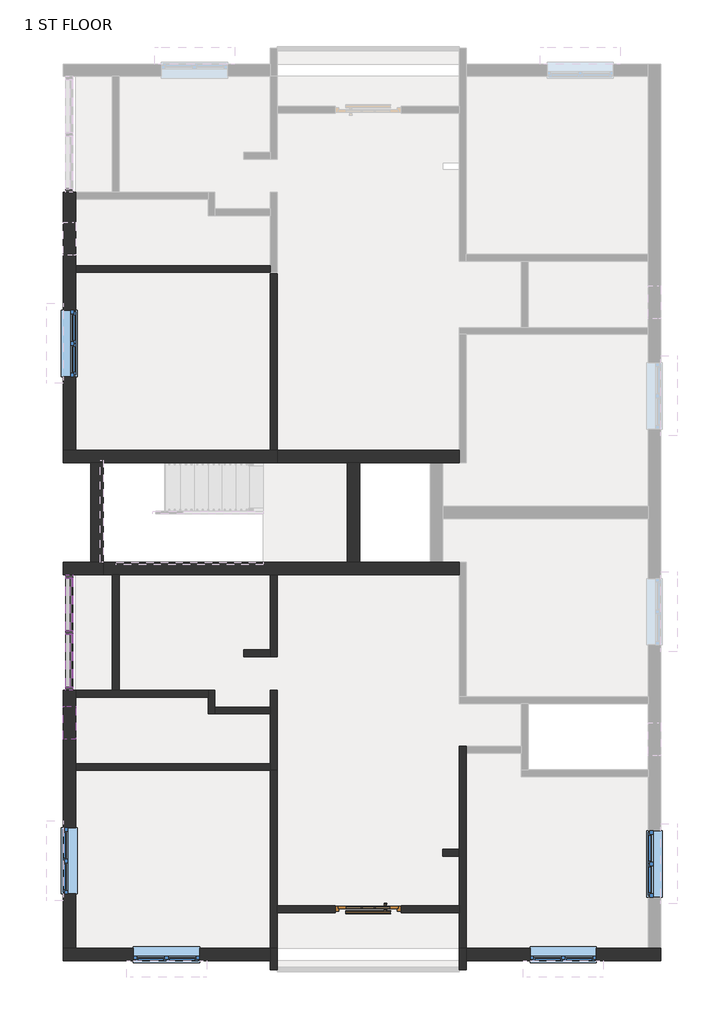
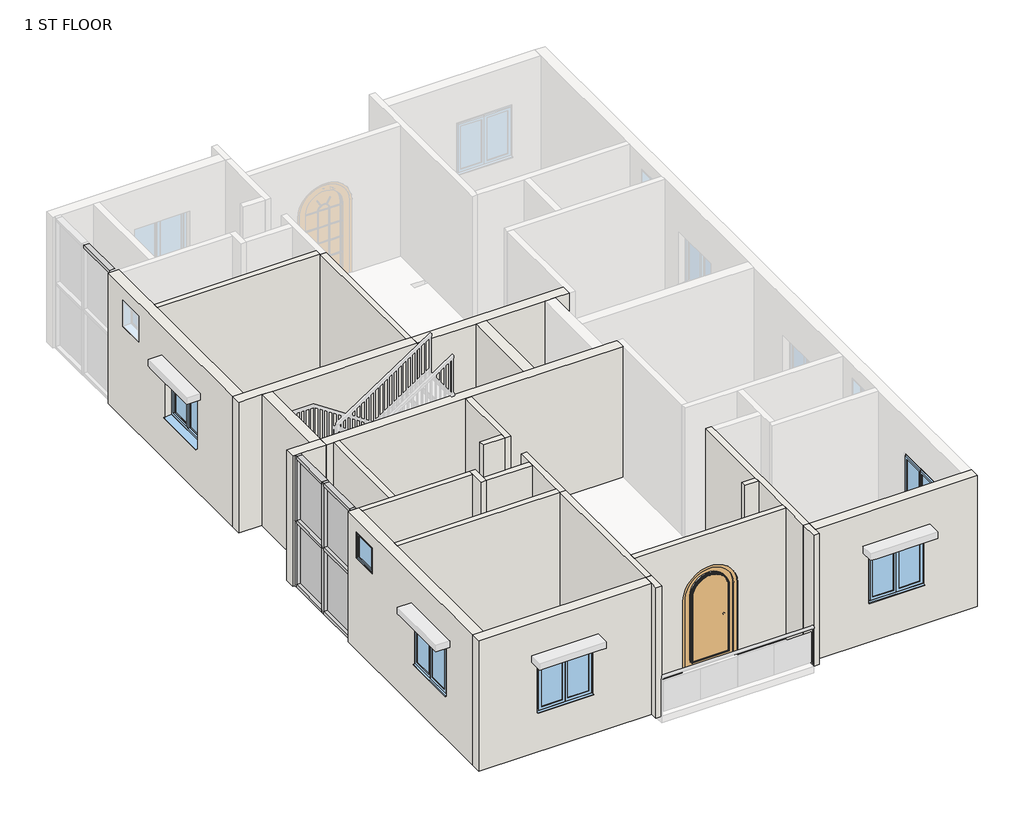
# One storey, part 1 of 4: 26 walls, 14 members, 6 windows, 4 plates, 1 door.
"""IFC4 building model written with IfcOpenShell, lengths in millimetres."""

from ifc_helpers import new_model, si_unit, point, frame, frame_2d, origin, place, context, project, spatial, polyline, circle_curve, trimmed, segment, composite_curve, outline, extrude, faceted_brep, transform, mapped, element, save
from components import door_arched_single_french_glass_wood_exterior_4_x_7_french_5c4dec95, member_801a2072, member_82905deb, member_88aa5c81, member_4491d118, system_panel_glazed_a8655be6, window_80340324, w2_windows_4_x_4_9dec5fc7

model = new_model("IFC4")

# Units and contexts
model_context = context("Model", 3, world=origin())
ifc_project = project(units=[si_unit("LENGTHUNIT", "METRE", prefix="MILLI")], contexts=[model_context])

# Site, building, storey
site = spatial("IfcSite", under=ifc_project)
building = spatial("IfcBuilding", under=site)
storey = spatial("IfcBuildingStorey", under=building, Name="1 ST FLOOR", Elevation=6096.0)

# Door
placement = place(None, origin())
door_arched_single_french_glass_wood_exterior_4_x_7_french_shape = door_arched_single_french_glass_wood_exterior_4_x_7_french_5c4dec95(model_context)
element("IfcDoor", 1, ObjectType="Door_Arched_Single_French_Glass_Wood_Exterior : 4' x 7' french door", at=placement, inside=storey, context=model_context, shape_type="MappedRepresentation", body=[
    mapped(door_arched_single_french_glass_wood_exterior_4_x_7_french_shape, transform((-817.6012202, -2286.2690997, 6096.0), x_axis=(-1.0, 0.0, 0.0), y_axis=(0.0, -1.0, 0.0), z_axis=(0.0, 0.0, 1.0))),
])

# Members
member_shape = member_801a2072(model_context)
element("IfcMember", 2, ObjectType="Rectangular Mullion : 2.5\" x 5\" rectangular", at=placement, inside=storey, context=model_context, shape_type="MappedRepresentation", body=[
    mapped(member_shape, transform((-6318.2887202, 10972.5309003, 9144.0), x_axis=(0.0, 0.0, 1.0), y_axis=(-1.0, 0.0, 0.0), z_axis=(0.0, -1.0, 0.0))),
])
element("IfcMember", 3, ObjectType="Rectangular Mullion : 2.5\" x 5\" rectangular", at=placement, inside=storey, context=model_context, shape_type="MappedRepresentation", body=[
    mapped(member_shape, transform((-6318.2887202, 1803.1309003, 9144.0), x_axis=(0.0, 0.0, 1.0), y_axis=(-1.0, 0.0, 0.0), z_axis=(0.0, -1.0, 0.0))),
])
element("IfcMember", 4, ObjectType="Rectangular Mullion : 2.5\" x 5\" rectangular", at=placement, inside=storey, context=model_context, shape_type="MappedRepresentation", body=[
    mapped(member_shape, transform((-6318.2887202, 2838.1809003, 9144.0), x_axis=(0.0, 0.0, 1.0), y_axis=(-1.0, 0.0, 0.0), z_axis=(0.0, -1.0, 0.0))),
])
element("IfcMember", 5, ObjectType="Rectangular Mullion : 2.5\" x 5\" rectangular", at=placement, inside=storey, context=model_context, shape_type="MappedRepresentation", body=[
    mapped(member_shape, transform((-6318.2887202, 3809.7309003, 6096.0), x_axis=(0.0, 0.0, -1.0), y_axis=(-1.0, 0.0, 0.0), z_axis=(0.0, 1.0, 0.0))),
])
element("IfcMember", 6, ObjectType="Rectangular Mullion : 2.5\" x 5\" rectangular", at=placement, inside=storey, context=model_context, shape_type="MappedRepresentation", body=[
    mapped(member_shape, transform((-6318.2887202, 2774.6809003, 6096.0), x_axis=(0.0, 0.0, -1.0), y_axis=(-1.0, 0.0, 0.0), z_axis=(0.0, 1.0, 0.0))),
])
member_2_shape = member_82905deb(model_context)
element("IfcMember", 7, ObjectType="Rectangular Mullion : 2.5\" x 5\" rectangular", at=placement, inside=storey, context=model_context, shape_type="MappedRepresentation", body=[
    mapped(member_2_shape, transform((-6318.2887202, 2806.4309003, 6096.0), x_axis=(0.0, -1.0, 0.0), y_axis=(-1.0, 0.0, 0.0), z_axis=(0.0, 0.0, -1.0))),
])
member_3_shape = member_88aa5c81(model_context)
element("IfcMember", 8, ObjectType="Rectangular Mullion : 2.5\" x 5\" rectangular", at=placement, inside=storey, context=model_context, shape_type="MappedRepresentation", body=[
    mapped(member_3_shape, transform((-6318.2887202, 2838.1809003, 7620.0), x_axis=(0.0, 0.0, 1.0), y_axis=(-1.0, 0.0, 0.0), z_axis=(0.0, -1.0, 0.0))),
])
element("IfcMember", 9, ObjectType="Rectangular Mullion : 2.5\" x 5\" rectangular", at=placement, inside=storey, context=model_context, shape_type="MappedRepresentation", body=[
    mapped(member_3_shape, transform((-6318.2887202, 1803.1309003, 7620.0), x_axis=(0.0, 0.0, 1.0), y_axis=(-1.0, 0.0, 0.0), z_axis=(0.0, -1.0, 0.0))),
])
element("IfcMember", 10, ObjectType="Rectangular Mullion : 2.5\" x 5\" rectangular", at=placement, inside=storey, context=model_context, shape_type="MappedRepresentation", body=[
    mapped(member_2_shape, transform((-6318.2887202, 2806.4309003, 7620.0), x_axis=(0.0, -1.0, 0.0), y_axis=(-1.0, 0.0, 0.0), z_axis=(0.0, 0.0, -1.0))),
])
member_4_shape = member_4491d118(model_context)
element("IfcMember", 11, ObjectType="Rectangular Mullion : 2.5\" x 5\" rectangular", at=placement, inside=storey, context=model_context, shape_type="MappedRepresentation", body=[
    mapped(member_4_shape, transform((-6318.2887202, 10909.0309003, 6096.0), x_axis=(0.0, -1.0, 0.0), y_axis=(-1.0, 0.0, 0.0), z_axis=(0.0, 0.0, -1.0))),
])
element("IfcMember", 12, ObjectType="Rectangular Mullion : 2.5\" x 5\" rectangular", at=placement, inside=storey, context=model_context, shape_type="MappedRepresentation", body=[
    mapped(member_4_shape, transform((-6318.2887202, 1739.6309003, 6096.0), x_axis=(0.0, -1.0, 0.0), y_axis=(-1.0, 0.0, 0.0), z_axis=(0.0, 0.0, -1.0))),
])
element("IfcMember", 13, ObjectType="Rectangular Mullion : 2.5\" x 5\" rectangular", at=placement, inside=storey, context=model_context, shape_type="MappedRepresentation", body=[
    mapped(member_4_shape, transform((-6318.2887202, 3873.2309003, 9144.0), x_axis=(0.0, 1.0, 0.0), y_axis=(-1.0, 0.0, 0.0), z_axis=(0.0, 0.0, 1.0))),
])
element("IfcMember", 14, ObjectType="Rectangular Mullion : 2.5\" x 5\" rectangular", at=placement, inside=storey, context=model_context, shape_type="MappedRepresentation", body=[
    mapped(member_4_shape, transform((-6318.2887202, 1739.6309003, 7620.0), x_axis=(0.0, -1.0, 0.0), y_axis=(-1.0, 0.0, 0.0), z_axis=(0.0, 0.0, -1.0))),
])
element("IfcMember", 15, ObjectType="Rectangular Mullion : 2.5\" x 5\" rectangular", at=placement, inside=storey, context=model_context, shape_type="MappedRepresentation", body=[
    mapped(member_4_shape, transform((-6318.2887202, 3873.2309003, 7620.0), x_axis=(0.0, 1.0, 0.0), y_axis=(-1.0, 0.0, 0.0), z_axis=(0.0, 0.0, 1.0))),
])

# Plates
system_panel_glazed_shape = system_panel_glazed_a8655be6(model_context)
element("IfcPlate", 16, ObjectType="System Panel : Glazed", at=placement, inside=storey, context=model_context, shape_type="MappedRepresentation", body=[
    mapped(system_panel_glazed_shape, transform((-6318.2887202, 3323.9559003, 6159.5), x_axis=(0.0, -1.0, 0.0), y_axis=(1.0, 0.0, 0.0), z_axis=(0.0, 0.0, 1.0))),
])
element("IfcPlate", 17, ObjectType="System Panel : Glazed", at=placement, inside=storey, context=model_context, shape_type="MappedRepresentation", body=[
    mapped(system_panel_glazed_shape, transform((-6318.2887202, 2288.9059003, 6159.5), x_axis=(0.0, -1.0, 0.0), y_axis=(1.0, 0.0, 0.0), z_axis=(0.0, 0.0, 1.0))),
])
element("IfcPlate", 18, ObjectType="System Panel : Glazed", at=placement, inside=storey, context=model_context, shape_type="MappedRepresentation", body=[
    mapped(system_panel_glazed_shape, transform((-6318.2887202, 3323.9559003, 7651.75), x_axis=(0.0, -1.0, 0.0), y_axis=(1.0, 0.0, 0.0), z_axis=(0.0, 0.0, 1.0))),
])
element("IfcPlate", 19, ObjectType="System Panel : Glazed", at=placement, inside=storey, context=model_context, shape_type="MappedRepresentation", body=[
    mapped(system_panel_glazed_shape, transform((-6318.2887202, 2288.9059003, 7651.75), x_axis=(0.0, -1.0, 0.0), y_axis=(1.0, 0.0, 0.0), z_axis=(0.0, 0.0, 1.0))),
])

# Walls
element("IfcWall", 20, ObjectType="OUTER WALL 9\"", at=placement, inside=storey, context=model_context, shape_type="Brep", body=[
    faceted_brep([(-6432.5887202, -3238.7690997, 6096.0), (-2621.0012202, -3238.7690997, 6096.0), (-2621.0012202, -3238.7690997, 9144.0), (-6432.5887202, -3238.7690997, 9144.0), (-5137.1887202, -3238.7690997, 7010.4), (-5137.1887202, -3238.7690997, 8229.6), (-3917.9887202, -3238.7690997, 8229.6), (-3917.9887202, -3238.7690997, 7010.4), (-6432.5887202, -3010.1690997, 6096.0), (-6432.5887202, -3010.1690997, 9144.0), (-6203.9887202, -3010.1690997, 9144.0), (-2621.0012202, -3010.1690997, 9144.0), (-2621.0012202, -3010.1690997, 6096.0), (-6203.9887202, -3010.1690997, 6096.0), (-5137.1887202, -3010.1690997, 7010.4), (-3917.9887202, -3010.1690997, 7010.4), (-3917.9887202, -3010.1690997, 8229.6), (-5137.1887202, -3010.1690997, 8229.6)], [[[0, 1, 2, 3], [4, 5, 6, 7]], [[8, 9, 10, 11, 12, 13], [14, 15, 16, 17]], [[1, 0, 8, 13, 12]], [[3, 2, 11, 10, 9]], [[0, 3, 9, 8]], [[2, 1, 12, 11]], [[5, 4, 14, 17]], [[6, 5, 17, 16]], [[7, 6, 16, 15]], [[4, 7, 15, 14]]]),
])
element("IfcWall", 21, ObjectType="OUTER WALL 9\"", at=placement, inside=storey, context=model_context, shape_type="Brep", body=[
    faceted_brep([(-6203.9887202, -3010.1690997, 9144.0), (-6203.9887202, -3010.1690997, 6096.0), (-6203.9887202, 266.4309003, 6096.0), (-6203.9887202, 393.4309003, 6096.0), (-6203.9887202, 1612.6309003, 6096.0), (-6203.9887202, 1739.6309003, 6096.0), (-6203.9887202, 1739.6309003, 9144.0), (-6203.9887202, 1612.6309003, 9144.0), (-6203.9887202, 393.4309003, 9144.0), (-6203.9887202, 266.4309003, 9144.0), (-6203.9887202, -787.6690997, 7096.0), (-6203.9887202, -2006.8690997, 7096.0), (-6203.9887202, -2006.8690997, 8315.2), (-6203.9887202, -787.6690997, 8315.2), (-6203.9887202, 1447.5309003, 8839.2), (-6203.9887202, 1447.5309003, 8229.6), (-6203.9887202, 837.9309003, 8229.6), (-6203.9887202, 837.9309003, 8839.2), (-6432.5887202, -3010.1690997, 6096.0), (-6432.5887202, -3010.1690997, 9144.0), (-6432.5887202, 1739.6309003, 9144.0), (-6432.5887202, 1739.6309003, 6096.0), (-6432.5887202, -787.6690997, 7096.0), (-6432.5887202, -787.6690997, 8315.2), (-6432.5887202, -2006.8690997, 8315.2), (-6432.5887202, -2006.8690997, 7096.0), (-6432.5887202, 1447.5309003, 8839.2), (-6432.5887202, 837.9309003, 8839.2), (-6432.5887202, 837.9309003, 8229.6), (-6432.5887202, 1447.5309003, 8229.6)], [[[0, 1, 2, 3, 4, 5, 6, 7, 8, 9], [10, 11, 12, 13], [14, 15, 16, 17]], [[18, 19, 20, 21], [22, 23, 24, 25], [26, 27, 28, 29]], [[1, 18, 21, 5, 4, 3, 2]], [[19, 0, 9, 8, 7, 6, 20]], [[1, 0, 19, 18]], [[6, 5, 21, 20]], [[23, 22, 10, 13]], [[24, 23, 13, 12]], [[25, 24, 12, 11]], [[22, 25, 11, 10]], [[15, 14, 26, 29]], [[16, 15, 29, 28]], [[17, 16, 28, 27]], [[14, 17, 27, 26]]]),
])
element("IfcWall", 22, ObjectType="OUTER WALL 9\"", at=placement, inside=storey, context=model_context, shape_type="Brep", body=[
    faceted_brep([(4567.1987798, -3010.1690997, 6096.0), (4338.5987798, -3010.1690997, 6096.0), (985.7987798, -3010.1690997, 6096.0), (985.7987798, -3010.1690997, 9144.0), (4338.5987798, -3010.1690997, 9144.0), (4567.1987798, -3010.1690997, 9144.0), (2166.8987798, -3010.1690997, 7010.4), (3386.0987798, -3010.1690997, 7010.4), (3386.0987798, -3010.1690997, 8229.6), (2166.8987798, -3010.1690997, 8229.6), (4567.1987798, -3238.7690997, 6096.0), (4567.1987798, -3238.7690997, 9144.0), (985.7987798, -3238.7690997, 9144.0), (985.7987798, -3238.7690997, 6096.0), (2166.8987798, -3238.7690997, 7010.4), (2166.8987798, -3238.7690997, 8229.6), (3386.0987798, -3238.7690997, 8229.6), (3386.0987798, -3238.7690997, 7010.4)], [[[0, 1, 2, 3, 4, 5], [6, 7, 8, 9]], [[10, 11, 12, 13], [14, 15, 16, 17]], [[2, 1, 0, 10, 13]], [[5, 4, 3, 12, 11]], [[0, 5, 11, 10]], [[15, 14, 6, 9]], [[16, 15, 9, 8]], [[17, 16, 8, 7]], [[14, 17, 7, 6]], [[3, 2, 13, 12]]]),
])
element("IfcWall", 23, ObjectType="OUTER WALL 9\"", at=placement, inside=storey, context=model_context, shape_type="SweptSolid", body=[
    extrude(outline(polyline([(6159.2309003, 6096.0), (6159.2309003, 9144.0), (10909.0309003, 9144.0), (10909.0309003, 6096.0), (6159.2309003, 6096.0)]), holes=[polyline([(7518.1309003, 7096.0), (8737.3309003, 7096.0), (8737.3309003, 8315.2), (7518.1309003, 8315.2), (7518.1309003, 7096.0)]), polyline([(9753.3309003, 8839.2), (9753.3309003, 8229.6), (10362.9309003, 8229.6), (10362.9309003, 8839.2), (9753.3309003, 8839.2)])]), frame((-6432.5887202, 0.0, 0.0), z_axis=(1.0, 0.0, 0.0), x_axis=(0.0, 1.0, 0.0)), (0.0, 0.0, 1.0), 228.6),
])
element("IfcWall", 24, ObjectType="OUTER WALL 9\"", at=placement, inside=storey, context=model_context, shape_type="Brep", body=[
    faceted_brep([(-6432.5887202, 5930.6309003, 6096.0), (-5923.0012202, 5930.6309003, 6096.0), (-5694.4012202, 5930.6309003, 6096.0), (-2494.0012202, 5930.6309003, 6096.0), (-2494.0012202, 5930.6309003, 9144.0), (-5694.4012202, 5930.6309003, 9144.0), (-5923.0012202, 5930.6309003, 9144.0), (-6432.5887202, 5930.6309003, 9144.0), (-6432.5887202, 6159.2309003, 6096.0), (-6432.5887202, 6159.2309003, 9144.0), (-6203.9887202, 6159.2309003, 9144.0), (-2621.0012202, 6159.2309003, 9144.0), (-2494.0012202, 6159.2309003, 9144.0), (-2494.0012202, 6159.2309003, 6096.0), (-2621.0012202, 6159.2309003, 6096.0), (-6203.9887202, 6159.2309003, 6096.0)], [[[0, 1, 2, 3, 4, 5, 6, 7]], [[8, 9, 10, 11, 12, 13, 14, 15]], [[3, 2, 1, 0, 8, 15, 14, 13]], [[7, 6, 5, 4, 12, 11, 10, 9]], [[0, 7, 9, 8]], [[4, 3, 13, 12]]]),
])
element("IfcWall", 25, ObjectType="OUTER WALL 9\"", at=placement, inside=storey, context=model_context, shape_type="SweptSolid", body=[
    extrude(outline(polyline([(-5923.0012202, 4101.8309003), (-5923.0012202, 5930.6309003), (-5694.4012202, 5930.6309003), (-5694.4012202, 4101.8309003), (-5923.0012202, 4101.8309003)])), frame((0.0, 0.0, 6096.0), z_axis=(0.0, 0.0, 1.0), x_axis=(1.0, 0.0, 0.0)), (0.0, 0.0, 1.0), 3048.0),
])
element("IfcWall", 26, ObjectType="OUTER WALL 9\"", at=placement, inside=storey, context=model_context, shape_type="Brep", body=[
    faceted_brep([(-5694.4012202, 4101.8309003, 6096.0), (-5923.0012202, 4101.8309003, 6096.0), (-6432.5887202, 4101.8309003, 6096.0), (-6432.5887202, 4101.8309003, 9144.0), (-5923.0012202, 4101.8309003, 9144.0), (-5694.4012202, 4101.8309003, 9144.0), (-5694.4012202, 3873.2309003, 6096.0), (-5694.4012202, 3873.2309003, 9144.0), (-6203.9887202, 3873.2309003, 9144.0), (-6432.5887202, 3873.2309003, 9144.0), (-6432.5887202, 3873.2309003, 6096.0), (-6203.9887202, 3873.2309003, 6096.0)], [[[0, 1, 2, 3, 4, 5]], [[6, 7, 8, 9, 10, 11]], [[2, 1, 0, 6, 11, 10]], [[5, 4, 3, 9, 8, 7]], [[0, 5, 7, 6]], [[3, 2, 10, 9]]]),
])
element("IfcWall", 27, ObjectType="OUTER WALL 9\"", at=placement, inside=storey, context=model_context, shape_type="Brep", body=[
    faceted_brep([(-5694.4012202, 3873.2309003, 6096.0), (-5529.3012202, 3873.2309003, 6096.0), (-5402.3012202, 3873.2309003, 6096.0), (-2621.0012202, 3873.2309003, 6096.0), (-2494.0012202, 3873.2309003, 6096.0), (858.7987798, 3873.2309003, 6096.0), (858.7987798, 3873.2309003, 9144.0), (-2494.0012202, 3873.2309003, 9144.0), (-2621.0012202, 3873.2309003, 9144.0), (-5402.3012202, 3873.2309003, 9144.0), (-5529.3012202, 3873.2309003, 9144.0), (-5694.4012202, 3873.2309003, 9144.0), (-5694.4012202, 4101.8309003, 6096.0), (-5694.4012202, 4101.8309003, 9144.0), (-1198.6012202, 4101.8309003, 9144.0), (-970.0012202, 4101.8309003, 9144.0), (325.3987798, 4101.8309003, 9144.0), (553.9987798, 4101.8309003, 9144.0), (858.7987798, 4101.8309003, 9144.0), (858.7987798, 4101.8309003, 6096.0), (553.9987798, 4101.8309003, 6096.0), (325.3987798, 4101.8309003, 6096.0), (-970.0012202, 4101.8309003, 6096.0), (-1198.6012202, 4101.8309003, 6096.0)], [[[0, 1, 2, 3, 4, 5, 6, 7, 8, 9, 10, 11]], [[12, 13, 14, 15, 16, 17, 18, 19, 20, 21, 22, 23]], [[5, 4, 3, 2, 1, 0, 12, 23, 22, 21, 20, 19]], [[11, 10, 9, 8, 7, 6, 18, 17, 16, 15, 14, 13]], [[0, 11, 13, 12]], [[6, 5, 19, 18]]]),
])
element("IfcWall", 28, ObjectType="OUTER WALL 9\"", at=placement, inside=storey, context=model_context, shape_type="Brep", body=[
    faceted_brep([(858.7987798, 6159.2309003, 6096.0), (-2494.0012202, 6159.2309003, 6096.0), (-2494.0012202, 6159.2309003, 9144.0), (858.7987798, 6159.2309003, 9144.0), (858.7987798, 5930.6309003, 6096.0), (858.7987798, 5930.6309003, 9144.0), (553.9987798, 5930.6309003, 9144.0), (325.3987798, 5930.6309003, 9144.0), (-970.0012202, 5930.6309003, 9144.0), (-1198.6012202, 5930.6309003, 9144.0), (-2494.0012202, 5930.6309003, 9144.0), (-2494.0012202, 5930.6309003, 6096.0), (-1198.6012202, 5930.6309003, 6096.0), (-970.0012202, 5930.6309003, 6096.0), (325.3987798, 5930.6309003, 6096.0), (553.9987798, 5930.6309003, 6096.0)], [[[0, 1, 2, 3]], [[4, 5, 6, 7, 8, 9, 10, 11, 12, 13, 14, 15]], [[1, 0, 4, 15, 14, 13, 12, 11]], [[3, 2, 10, 9, 8, 7, 6, 5]], [[2, 1, 11, 10]], [[0, 3, 5, 4]]]),
])
element("IfcWall", 29, ObjectType="OUTER WALL 9\"", at=placement, inside=storey, context=model_context, shape_type="SweptSolid", body=[
    extrude(outline(polyline([(-1198.6012202, 4101.8309003), (-1198.6012202, 5930.6309003), (-970.0012202, 5930.6309003), (-970.0012202, 4101.8309003), (-1198.6012202, 4101.8309003)])), frame((0.0, 0.0, 6096.0), z_axis=(0.0, 0.0, 1.0), x_axis=(1.0, 0.0, 0.0)), (0.0, 0.0, 1.0), 3048.0),
])
element("IfcWall", 30, ObjectType="inner wall 5\"", at=placement, inside=storey, context=model_context, shape_type="SweptSolid", body=[
    extrude(outline(polyline([(-6202.4012202, 9562.8309003), (-2621.0012202, 9562.8309003), (-2621.0012202, 9435.8309003), (-6202.4012202, 9435.8309003), (-6202.4012202, 9562.8309003)])), frame((0.0, 0.0, 6096.0), z_axis=(0.0, 0.0, 1.0), x_axis=(1.0, 0.0, 0.0)), (0.0, 0.0, 1.0), 3048.0),
])
element("IfcWall", 31, ObjectType="inner wall 5\"", at=placement, inside=storey, context=model_context, shape_type="SweptSolid", body=[
    extrude(outline(polyline([(-5529.3012202, 1739.6309003), (-5529.3012202, 3873.2309003), (-5402.3012202, 3873.2309003), (-5402.3012202, 1739.6309003), (-5529.3012202, 1739.6309003)])), frame((0.0, 0.0, 6096.0), z_axis=(0.0, 0.0, 1.0), x_axis=(1.0, 0.0, 0.0)), (0.0, 0.0, 1.0), 3048.0),
])
element("IfcWall", 32, ObjectType="inner wall 5\"", at=placement, inside=storey, context=model_context, shape_type="Brep", body=[
    faceted_brep([(-2621.0012202, 3873.2309003, 6096.0), (-2621.0012202, 2488.9309003, 6096.0), (-2621.0012202, 2361.9309003, 6096.0), (-2621.0012202, 2361.9309003, 9144.0), (-2621.0012202, 2488.9309003, 9144.0), (-2621.0012202, 3873.2309003, 9144.0), (-2494.0012202, 3873.2309003, 6096.0), (-2494.0012202, 3873.2309003, 9144.0), (-2494.0012202, 2361.9309003, 9144.0), (-2494.0012202, 2361.9309003, 6096.0)], [[[0, 1, 2, 3, 4, 5]], [[6, 7, 8, 9]], [[2, 1, 0, 6, 9]], [[5, 4, 3, 8, 7]], [[0, 5, 7, 6]], [[3, 2, 9, 8]]]),
])
element("IfcWall", 33, ObjectType="inner wall 5\"", at=placement, inside=storey, context=model_context, shape_type="SweptSolid", body=[
    extrude(outline(polyline([(-3103.6012202, 2488.9309003), (-2621.0012202, 2488.9309003), (-2621.0012202, 2361.9309003), (-3103.6012202, 2361.9309003), (-3103.6012202, 2488.9309003)])), frame((0.0, 0.0, 6096.0), z_axis=(0.0, 0.0, 1.0), x_axis=(1.0, 0.0, 0.0)), (0.0, 0.0, 1.0), 3048.0),
])
element("IfcWall", 34, ObjectType="inner wall 5\"", at=placement, inside=storey, context=model_context, shape_type="Brep", body=[
    faceted_brep([(-6203.9887202, 1612.6309003, 6096.0), (-3764.0012202, 1612.6309003, 6096.0), (-3764.0012202, 1612.6309003, 9144.0), (-6203.9887202, 1612.6309003, 9144.0), (-6203.9887202, 1739.6309003, 6096.0), (-6203.9887202, 1739.6309003, 9144.0), (-5529.3012202, 1739.6309003, 9144.0), (-5402.3012202, 1739.6309003, 9144.0), (-3764.0012202, 1739.6309003, 9144.0), (-3764.0012202, 1739.6309003, 6096.0), (-5402.3012202, 1739.6309003, 6096.0), (-5529.3012202, 1739.6309003, 6096.0)], [[[0, 1, 2, 3]], [[4, 5, 6, 7, 8, 9, 10, 11]], [[1, 0, 4, 11, 10, 9]], [[3, 2, 8, 7, 6, 5]], [[0, 3, 5, 4]], [[2, 1, 9, 8]]]),
])
element("IfcWall", 35, ObjectType="inner wall 5\"", at=placement, inside=storey, context=model_context, shape_type="Brep", body=[
    faceted_brep([(-3764.0012202, 1739.6309003, 6096.0), (-3764.0012202, 1612.6309003, 6096.0), (-3764.0012202, 1307.8309003, 6096.0), (-3764.0012202, 1307.8309003, 9144.0), (-3764.0012202, 1612.6309003, 9144.0), (-3764.0012202, 1739.6309003, 9144.0), (-3637.0012202, 1739.6309003, 6096.0), (-3637.0012202, 1739.6309003, 9144.0), (-3637.0012202, 1434.8309003, 9144.0), (-3637.0012202, 1307.8309003, 9144.0), (-3637.0012202, 1307.8309003, 6096.0), (-3637.0012202, 1434.8309003, 6096.0)], [[[0, 1, 2, 3, 4, 5]], [[6, 7, 8, 9, 10, 11]], [[2, 1, 0, 6, 11, 10]], [[5, 4, 3, 9, 8, 7]], [[0, 5, 7, 6]], [[3, 2, 10, 9]]]),
])
element("IfcWall", 36, ObjectType="inner wall 5\"", at=placement, inside=storey, context=model_context, shape_type="SweptSolid", body=[
    extrude(outline(polyline([(-2621.0012202, 1307.8309003), (-3637.0012202, 1307.8309003), (-3637.0012202, 1434.8309003), (-2621.0012202, 1434.8309003), (-2621.0012202, 1307.8309003)])), frame((0.0, 0.0, 6096.0), z_axis=(0.0, 0.0, 1.0), x_axis=(1.0, 0.0, 0.0)), (0.0, 0.0, 1.0), 3048.0),
])
element("IfcWall", 37, ObjectType="inner wall 5\"", at=placement, inside=storey, context=model_context, shape_type="Brep", body=[
    faceted_brep([(-2621.0012202, 1739.6309003, 6096.0), (-2621.0012202, 1434.8309003, 6096.0), (-2621.0012202, 1307.8309003, 6096.0), (-2621.0012202, 393.4309003, 6096.0), (-2621.0012202, 266.4309003, 6096.0), (-2621.0012202, 266.4309003, 9144.0), (-2621.0012202, 393.4309003, 9144.0), (-2621.0012202, 1307.8309003, 9144.0), (-2621.0012202, 1434.8309003, 9144.0), (-2621.0012202, 1739.6309003, 9144.0), (-2494.0012202, 1739.6309003, 6096.0), (-2494.0012202, 1739.6309003, 9144.0), (-2494.0012202, 266.4309003, 9144.0), (-2494.0012202, 266.4309003, 6096.0)], [[[0, 1, 2, 3, 4, 5, 6, 7, 8, 9]], [[10, 11, 12, 13]], [[4, 3, 2, 1, 0, 10, 13]], [[9, 8, 7, 6, 5, 12, 11]], [[0, 9, 11, 10]], [[5, 4, 13, 12]]]),
])
element("IfcWall", 38, ObjectType="inner wall 5\"", at=placement, inside=storey, context=model_context, shape_type="SweptSolid", body=[
    extrude(outline(polyline([(-6203.9887202, 393.4309003), (-2621.0012202, 393.4309003), (-2621.0012202, 266.4309003), (-6203.9887202, 266.4309003), (-6203.9887202, 393.4309003)])), frame((0.0, 0.0, 6096.0), z_axis=(0.0, 0.0, 1.0), x_axis=(1.0, 0.0, 0.0)), (0.0, 0.0, 1.0), 3048.0),
])
element("IfcWall", 39, ObjectType="inner wall 5\"", at=placement, inside=storey, context=model_context, shape_type="Brep", body=[
    faceted_brep([(-2494.0012202, -3010.1690997, 6096.0), (-2494.0012202, -2349.7690997, 6096.0), (-2494.0012202, -2222.7690997, 6096.0), (-2494.0012202, 266.4309003, 6096.0), (-2494.0012202, 266.4309003, 9144.0), (-2494.0012202, -2222.7690997, 9144.0), (-2494.0012202, -2349.7690997, 9144.0), (-2494.0012202, -3010.1690997, 9144.0), (-2621.0012202, -3010.1690997, 6096.0), (-2621.0012202, -3010.1690997, 9144.0), (-2621.0012202, 266.4309003, 9144.0), (-2621.0012202, 266.4309003, 6096.0)], [[[0, 1, 2, 3, 4, 5, 6, 7]], [[8, 9, 10, 11]], [[3, 2, 1, 0, 8, 11]], [[7, 6, 5, 4, 10, 9]], [[4, 3, 11, 10]], [[0, 7, 9, 8]]]),
])
element("IfcWall", 40, ObjectType="inner wall 5\"", at=placement, inside=storey, context=model_context, shape_type="Brep", body=[
    faceted_brep([(985.7987798, -3010.1690997, 6096.0), (985.7987798, 583.9309003, 6096.0), (985.7987798, 710.9309003, 6096.0), (985.7987798, 710.9309003, 9144.0), (985.7987798, 583.9309003, 9144.0), (985.7987798, -3010.1690997, 9144.0), (858.7987798, -3010.1690997, 6096.0), (858.7987798, -3010.1690997, 9144.0), (858.7987798, -2349.7690997, 9144.0), (858.7987798, -2222.7690997, 9144.0), (858.7987798, -1308.3690997, 9144.0), (858.7987798, -1181.3690997, 9144.0), (858.7987798, 710.9309003, 9144.0), (858.7987798, 710.9309003, 6096.0), (858.7987798, -1181.3690997, 6096.0), (858.7987798, -1308.3690997, 6096.0), (858.7987798, -2222.7690997, 6096.0), (858.7987798, -2349.7690997, 6096.0)], [[[0, 1, 2, 3, 4, 5]], [[6, 7, 8, 9, 10, 11, 12, 13, 14, 15, 16, 17]], [[2, 1, 0, 6, 17, 16, 15, 14, 13]], [[5, 4, 3, 12, 11, 10, 9, 8, 7]], [[3, 2, 13, 12]], [[0, 5, 7, 6]]]),
])
element("IfcWall", 41, ObjectType="inner wall 5\"", at=placement, inside=storey, context=model_context, shape_type="Brep", body=[
    faceted_brep([(-2621.0012202, -3010.1690997, 6096.0), (-2621.0012202, -3238.7690997, 6096.0), (-2621.0012202, -3403.8690997, 6096.0), (-2621.0012202, -3403.8690997, 9144.0), (-2621.0012202, -3238.7690997, 9144.0), (-2621.0012202, -3010.1690997, 9144.0), (-2494.0012202, -3010.1690997, 6096.0), (-2494.0012202, -3010.1690997, 9144.0), (-2494.0012202, -3403.8690997, 9144.0), (-2494.0012202, -3403.8690997, 6096.0)], [[[0, 1, 2, 3, 4, 5]], [[6, 7, 8, 9]], [[2, 1, 0, 6, 9]], [[3, 2, 9, 8]], [[5, 4, 3, 8, 7]], [[0, 5, 7, 6]]]),
])
element("IfcWall", 42, ObjectType="inner wall 5\"", at=placement, inside=storey, context=model_context, shape_type="SweptSolid", body=[
    extrude(outline(composite_curve([segment(polyline([(6096.0, -2494.0012202), (6096.0, -1427.2012202), (7774.6, -1427.2012202)]), True, "CONTINUOUS"), segment(trimmed(circle_curve(frame_2d((7774.6, -817.6012202)), 609.6), [point((7774.6, -1427.2012202))], [point((7774.6, -208.0012202))], True, "CARTESIAN"), True, "CONTINUOUS"), segment(polyline([(7774.6, -208.0012202), (6096.0, -208.0012202), (6096.0, 858.7987798), (9144.0, 858.7987798), (9144.0, -2494.0012202), (6096.0, -2494.0012202)]), True, "CONTINUOUS")], self_intersect=False)), frame((0.0, -2349.7690997, 0.0), z_axis=(0.0, 1.0, 0.0), x_axis=(0.0, 0.0, 1.0)), (0.0, 0.0, 1.0), 127.0),
])
element("IfcWall", 43, ObjectType="inner wall 5\"", at=placement, inside=storey, context=model_context, shape_type="SweptSolid", body=[
    extrude(outline(polyline([(553.9987798, -1181.3690997), (858.7987798, -1181.3690997), (858.7987798, -1308.3690997), (553.9987798, -1308.3690997), (553.9987798, -1181.3690997)])), frame((0.0, 0.0, 6096.0), z_axis=(0.0, 0.0, 1.0), x_axis=(1.0, 0.0, 0.0)), (0.0, 0.0, 1.0), 3048.0),
])
element("IfcWall", 44, ObjectType="inner wall 5\"", at=placement, inside=storey, context=model_context, shape_type="SweptSolid", body=[
    extrude(outline(polyline([(-2621.0012202, 6159.2309003), (-2621.0012202, 9410.4309003), (-2494.0012202, 9410.4309003), (-2494.0012202, 6159.2309003), (-2621.0012202, 6159.2309003)])), frame((0.0, 0.0, 6096.0), z_axis=(0.0, 0.0, 1.0), x_axis=(1.0, 0.0, 0.0)), (0.0, 0.0, 1.0), 3048.0),
])
element("IfcWall", 45, ObjectType="inner wall 5\"", at=placement, inside=storey, context=model_context, shape_type="Brep", body=[
    faceted_brep([(858.7987798, -3010.1690997, 6096.0), (858.7987798, -3403.8690997, 6096.0), (858.7987798, -3403.8690997, 9144.0), (858.7987798, -3010.1690997, 9144.0), (985.7987798, -3010.1690997, 6096.0), (985.7987798, -3010.1690997, 9144.0), (985.7987798, -3238.7690997, 9144.0), (985.7987798, -3403.8690997, 9144.0), (985.7987798, -3403.8690997, 6096.0), (985.7987798, -3238.7690997, 6096.0)], [[[0, 1, 2, 3]], [[4, 5, 6, 7, 8, 9]], [[1, 0, 4, 9, 8]], [[2, 1, 8, 7]], [[3, 2, 7, 6, 5]], [[0, 3, 5, 4]]]),
])

# Windows
window_shape = window_80340324(model_context)
element("IfcWindow", 46, ObjectType="Fixed : 24\" x 24\"", at=placement, inside=storey, context=model_context, shape_type="MappedRepresentation", body=[
    mapped(window_shape, transform((-6318.2887202, 1180.8309003, 7315.2), x_axis=(0.0, 1.0, 0.0), y_axis=(-1.0, 0.0, 0.0), z_axis=(0.0, 0.0, 1.0))),
])
w2_windows_4_x_4_shape = w2_windows_4_x_4_9dec5fc7(model_context)
element("IfcWindow", 47, ObjectType="w2 : windows 4' x 4'", at=placement, inside=storey, context=model_context, shape_type="MappedRepresentation", body=[
    mapped(w2_windows_4_x_4_shape, transform((-4527.5887202, -3124.4690997, 6010.4), x_axis=(1.0, 0.0, 0.0), y_axis=(0.0, 1.0, 0.0), z_axis=(0.0, 0.0, 1.0))),
])
element("IfcWindow", 48, ObjectType="w2 : windows 4' x 4'", at=placement, inside=storey, context=model_context, shape_type="MappedRepresentation", body=[
    mapped(w2_windows_4_x_4_shape, transform((2776.4987798, -3124.4690997, 6010.4), x_axis=(1.0, 0.0, 0.0), y_axis=(0.0, 1.0, 0.0), z_axis=(0.0, 0.0, 1.0))),
])
element("IfcWindow", 49, ObjectType="w2 : windows 4' x 4'", at=placement, inside=storey, context=model_context, shape_type="MappedRepresentation", body=[
    mapped(w2_windows_4_x_4_shape, transform((-6318.2887202, 8127.7309003, 6096.0), x_axis=(0.0, 1.0, 0.0), y_axis=(-1.0, 0.0, 0.0), z_axis=(0.0, 0.0, 1.0))),
])
element("IfcWindow", 50, ObjectType="w2 : windows 4' x 4'", at=placement, inside=storey, context=model_context, shape_type="MappedRepresentation", body=[
    mapped(w2_windows_4_x_4_shape, transform((4452.8987798, -1454.4190997, 6096.0), x_axis=(0.0, -1.0, 0.0), y_axis=(1.0, 0.0, 0.0), z_axis=(0.0, 0.0, 1.0))),
])
element("IfcWindow", 51, ObjectType="w2 : windows 4' x 4'", at=placement, inside=storey, context=model_context, shape_type="MappedRepresentation", body=[
    mapped(w2_windows_4_x_4_shape, transform((-6318.2887202, -1397.2690997, 6096.0), x_axis=(0.0, -1.0, 0.0), y_axis=(1.0, 0.0, 0.0), z_axis=(0.0, 0.0, 1.0))),
])

save(model, "model.ifc")

# Revit data of these elements
# Type "Door_Arched_Single_French_Glass_Wood_Exterior : 4' x 7' french door"
#   Type Mark = "17"
#   Type Comments = "External Single"
#   Operation = "SingleSwingRight"
#   Keynote = "L20"
#   Analytic Construction = "<None>"
#   Wrap Layers (Int) from Ext = 0' - 6.98819"
#   Wrap Layers (Ext) from Ext = 0' - 4.03543"
#   Thickness = 0' - 1.73228"
#   Stile Shutting = 0' - 5.90551"
#   Stile - Top Rail = 0' - 5.90551"
#   Stile - Hanging = 0' - 5.90551"
#   Stile - Bottom Rail = 0' - 6.88976"
#   Rough Width = 4' - 0"
#   Rough Height = 7' - 0"
#   O/A Frame Width = 0' - 2.51969"
#   Handle Z Distance = 3' - 5.33858"
#   Glazing Thickness = 0' - 0.94488"
#   Glazing Bar Thickness = 0' - 0.7874"
#   FrameWidth = 0' - 1.65354"
#   FrameOffset - External = 0' - 0.98425"
#   FrameDepth = 0' - 3.50394"
#   Door Panel Width = 3' - 7.94488"
#   Handle X Distance = 0' - 2.95276"
#   Height = 7' - 0"
#   Structural Tolerance = 0' - 0.25591"
#   Tolerance = 0' - 0.11811"
#   Undercut = 0' - 0.15748"
#   Width = 4' - 0"
#   Door Panel Thickness = 0' - 1.73228"
#   Door Panel Height = 6' - 9.81496"
#   Cavity Closer Width = 0' - 1.9685"
#   Cavity Closer Offset from Ext = 0' - 4.03543"
#   Cavity Closer Depth = 0' - 3.34646"
#   Vis - Ironmongery = yes
#   Vis - Cavity Closers = yes
#   Define Thermal Properties by = 1
#   Material Glass = Door - Glazing
#   Handle Style = element 430241
#   Material Door = Door - Panel
#   Material Frame = BROWN
#   Material Ironmongery = Door - Handle
#   Function = (empty or 0)
#   Wall Closure = (empty or 0)
#   Assembly Code = ""
# Type "Rectangular Mullion : 2.5\" x 5\" rectangular"
#   built-in parameter 1007304 = 0.416667 (stored number, unit not read)
#   built-in parameter 1007301 = 0.104167 (stored number, unit not read)
#   built-in parameter 1007300 = 0.104167 (stored number, unit not read)
# Type "System Panel : Glazed"
#   Construction Type Id = "GSP4R"
#   Analytic Construction = "1/8 in Pilkington single glazing"
#   Visual Light Transmittance = 0.9
#   Solar Heat Gain Coefficient = 0.86
#   Heat Transfer Coefficient (U) = 1.18115 BTU/(h·ft²·°F)
#   Define Thermal Properties by = 1
# Type "OUTER WALL 9\""
#   Assembly Code = "B2010"
#   Layers, outside or top first: 0' - 9" "ROSE COLOUR" (function 1)
# Type "inner wall 5\""
#   Assembly Code = "B2010"
#   Layers, outside or top first: 0' - 5" "ROSE COLOUR" (function 1)
# Type "Fixed : 24\" x 24\""
#   Type Mark = "3"
#   Construction Type Id = "GSP4R"
#   Assembly Code = "B2020100"
#   Analytic Construction = "1/8 in Pilkington single glazing"
#   Visual Light Transmittance = 0.9
#   Solar Heat Gain Coefficient = 0.78
#   Heat Transfer Coefficient (U) = 0.6496 BTU/(h·ft²·°F)
#   Height = 2' - 0"
#   Default Sill Height = 3' - 0"
#   Width = 2' - 0"
#   Window Inset = 0' - 0 3/4"
#   Define Thermal Properties by = 1
#   Define Thermal Properties by = 1
#   Glass Pane Material = Glass
#   Sash Material = Sash
#   Wall Closure = (empty or 0)
# Type "w2 : windows 4' x 4'"
#   Type Mark = "31"
#   Operation = "DoublePanelVertical"
#   Keynote = "16.05.01"
#   Analytic Construction = "<None>"
#   Rough Width = 4' - 0"
#   Rough Height = 4' - 0"
#   Rahmentiefe = 0' - 2.3622"
#   Rahmenhöhe unten = 0' - 3.14961"
#   Rahmehöhe oben = 0' - 3.14961"
#   Rahmenbreite = 0' - 2.3622"
#   Heat Transfer Coefficient (U) = 2.81836 BTU/(h·ft²·°F)
#   Height = 4' - 0"
#   Flügeltiefe = 0' - 2.3622"
#   Flügelbreite = 0' - 2.3622"
#   Einbautiefe (von außen) [instance default] = 0' - 5.51181"
#   Width = 4' - 0"
#   Kippflügel [instance default] = yes
#   Drehflügel im Grundriß darstellen [instance default] = no
#   Drehflügel [instance default] = yes
#   Define Thermal Properties by = 1
#   Rahmen [instance default] = none
#   Glas [instance default] = blue glass
#   Flügel [instance default] = WINDOW COLOUR WHITE
#   Fensterbank aussen [instance default] = WINDOW COLOUR WHITE
#   Fensterbank innen [instance default] = WINDOW COLOUR WHITE
#   Visual Light Transmittance = 0
#   Thermal Resistance (R) = 0
#   Solar Heat Gain Coefficient = 0
#   Wall Closure = (empty or 0)
# Element 1 (IfcDoor, "Door_Arched_Single_French_Glass_Wood_Exterior : 4' x 7' french door")
#   Phase Created = New Construction
#   Materials on its faces: "Door - Panel", "Door - Handle", "BROWN", "Door - Glazing"
# Elements 2, 3, 4, 5, 6, 7, 8, 9, 10, 11, 12, 13, 14, 15 (IfcMember, "Rectangular Mullion : 2.5\" x 5\" rectangular")
#   Phase Created = New Construction
#   Materials on its faces: "Aluminum"
# Elements 16, 17, 18, 19 (IfcPlate, "System Panel : Glazed")
#   Phase Created = New Construction
#   Materials on its faces: "Glass"
# Elements 20, 21, 22, 23, 24, 25, 26, 27, 28, 29 (IfcWall, "OUTER WALL 9\"")
#   Top Offset = 0' - 0"
#   Base Offset = 0' - 0"
#   wall height = 10' - 0"
#   Phase Created = New Construction
#   Base Constraint = 1 ST FLOOR
#   Top Constraint = 2ND FLOOR
#   Materials on its faces: "ROSE COLOUR"
# Elements 30, 31, 32, 33, 34, 35, 36, 37, 38, 39, 40, 41, 42, 43, 44, 45 (IfcWall, "inner wall 5\"")
#   Top Offset = 0' - 0"
#   Base Offset = 0' - 0"
#   wall height = 10' - 0"
#   Phase Created = New Construction
#   Base Constraint = 1 ST FLOOR
#   Top Constraint = 2ND FLOOR
#   Materials on its faces: "ROSE COLOUR"
# Element 46 (IfcWindow, "Fixed : 24\" x 24\"")
#   Mark = "34"
#   Phase Created = New Construction
#   Materials on its faces: "Sash", "Glass"
# Element 47 (IfcWindow, "w2 : windows 4' x 4'")
#   Mark = "26"
#   Phase Created = New Construction
#   Materials on its faces: "WINDOW COLOUR WHITE", "blue glass"
# Element 48 (IfcWindow, "w2 : windows 4' x 4'")
#   Mark = "27"
#   Phase Created = New Construction
#   Materials on its faces: "WINDOW COLOUR WHITE", "blue glass"
# Element 49 (IfcWindow, "w2 : windows 4' x 4'")
#   Mark = "30"
#   Einbautiefe (von außen) = 0' - 5.51181"
#   Kippflügel = yes
#   Drehflügel im Grundriß darstellen = no
#   Drehflügel = yes
#   Rahmen = none
#   Glas = blue glass
#   Flügel = WINDOW COLOUR WHITE
#   Fensterbank innen = WINDOW COLOUR WHITE
#   Fensterbank aussen = WINDOW COLOUR WHITE
#   Phase Created = New Construction
#   Materials on its faces: "WINDOW COLOUR WHITE", "blue glass"
# Element 50 (IfcWindow, "w2 : windows 4' x 4'")
#   Mark = "31"
#   Einbautiefe (von außen) = 0' - 5.51181"
#   Kippflügel = yes
#   Drehflügel im Grundriß darstellen = no
#   Drehflügel = yes
#   Rahmen = none
#   Glas = blue glass
#   Flügel = WINDOW COLOUR WHITE
#   Fensterbank innen = WINDOW COLOUR WHITE
#   Fensterbank aussen = WINDOW COLOUR WHITE
#   Phase Created = New Construction
#   Materials on its faces: "WINDOW COLOUR WHITE", "blue glass"
# Element 51 (IfcWindow, "w2 : windows 4' x 4'")
#   Mark = "32"
#   Einbautiefe (von außen) = 0' - 5.51181"
#   Kippflügel = yes
#   Drehflügel im Grundriß darstellen = no
#   Drehflügel = yes
#   Rahmen = none
#   Glas = blue glass
#   Flügel = WINDOW COLOUR WHITE
#   Fensterbank innen = WINDOW COLOUR WHITE
#   Fensterbank aussen = WINDOW COLOUR WHITE
#   Phase Created = New Construction
#   Materials on its faces: "WINDOW COLOUR WHITE", "blue glass"
# Materials
#   "Door - Glazing": colour RGB 218 227 224, transparency 0.85
#   "Door - Panel": class "Wood", colour RGB 210 159 95, transparency 0, Cost = 0
#   "BROWN": class "Generic", colour RGB 120 120 120, transparency 0, Cost = 0
#   "Door - Handle": colour RGB 0 0 0, transparency 0, Keynote = "P21"
#   "ROSE COLOUR": class "Generic", colour RGB 120 120 120, transparency 0, Cost = 0
#   "Glass": class "Glass", colour RGB 0 128 192, transparency 0.75, Description = "Soda Lime Glass", Cost = 0
#   "Sash": class "Wood", colour RGB 224 178 126, transparency 0, Cost = 0
#   "blue glass": class "System", colour RGB 0 0 255, transparency 0.75, Cost = 0
#   "WINDOW COLOUR WHITE": class "Generic", colour RGB 120 120 120, transparency 0, Cost = 0
#   "Aluminum": class "Metal", colour RGB 247 247 247, transparency 0, Description = "Aluminum 6061", Cost = 0
